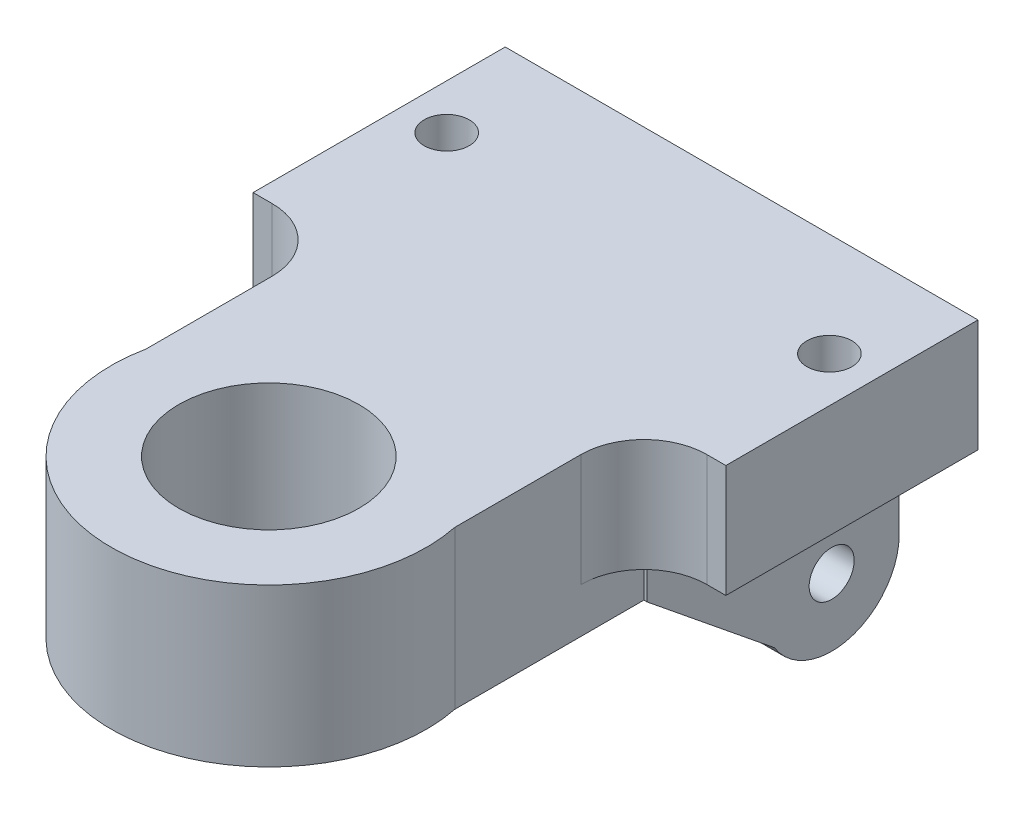
ISO-10303-21;
HEADER;
FILE_DESCRIPTION(('STEP AP214'),'2;1');
FILE_NAME('part.step','',(''),(''),'','','');
FILE_SCHEMA(('AUTOMOTIVE_DESIGN { 1 0 10303 214 1 1 1 1 }'));
ENDSEC;
DATA;
#1=APPLICATION_CONTEXT('core data for automotive mechanical design processes');
#2=APPLICATION_PROTOCOL_DEFINITION('international standard','automotive_design',2000,#1);
#3=PRODUCT_CONTEXT('',#1,'mechanical');
#4=PRODUCT('Part','Part','',(#3));
#5=PRODUCT_RELATED_PRODUCT_CATEGORY('part','',(#4));
#6=PRODUCT_DEFINITION_FORMATION('','',#4);
#7=PRODUCT_DEFINITION_CONTEXT('part definition',#1,'design');
#8=PRODUCT_DEFINITION('design','',#6,#7);
#9=PRODUCT_DEFINITION_SHAPE('','',#8);
#10=(LENGTH_UNIT() NAMED_UNIT(*) SI_UNIT(.MILLI.,.METRE.));
#11=(NAMED_UNIT(*) PLANE_ANGLE_UNIT() SI_UNIT($,.RADIAN.));
#12=(NAMED_UNIT(*) SI_UNIT($,.STERADIAN.) SOLID_ANGLE_UNIT());
#13=UNCERTAINTY_MEASURE_WITH_UNIT(LENGTH_MEASURE(1.E-05),#10,'distance_accuracy_value','');
#14=(GEOMETRIC_REPRESENTATION_CONTEXT(3) GLOBAL_UNCERTAINTY_ASSIGNED_CONTEXT((#13)) GLOBAL_UNIT_ASSIGNED_CONTEXT((#10,
#11,#12)) REPRESENTATION_CONTEXT('',''));
#15=CARTESIAN_POINT('',(0.,0.,0.));
#16=DIRECTION('',(0.,0.,1.));
#17=DIRECTION('',(1.,0.,0.));
#18=AXIS2_PLACEMENT_3D('',#15,#16,#17);
#19=CARTESIAN_POINT('',(0.,-22.5,0.));
#20=DIRECTION('',(0.,1.,0.));
#21=DIRECTION('',(0.,0.,1.));
#22=AXIS2_PLACEMENT_3D('',#19,#20,#21);
#23=PLANE('',#22);
#24=CARTESIAN_POINT('',(0.,-22.5,35.));
#25=DIRECTION('',(0.,1.,0.));
#26=DIRECTION('',(0.,0.,1.));
#27=AXIS2_PLACEMENT_3D('',#24,#25,#26);
#28=CIRCLE('',#27,20.);
#29=CARTESIAN_POINT('',(0.,-22.5,55.));
#30=VERTEX_POINT('',#29);
#31=EDGE_CURVE('E253',#30,#30,#28,.T.);
#32=ORIENTED_EDGE('',*,*,#31,.T.);
#33=EDGE_LOOP('',(#32));
#34=FACE_BOUND('',#33,.T.);
#35=DIRECTION('',(0.,0.,-1.));
#36=VECTOR('',#35,1.);
#37=CARTESIAN_POINT('',(-34.2928563989645,-22.5,-14.));
#38=LINE('',#37,#36);
#39=CARTESIAN_POINT('',(-34.2928563989645,-22.5,28.));
#40=VERTEX_POINT('',#39);
#41=CARTESIAN_POINT('',(-34.2928563989645,-22.5,-14.));
#42=VERTEX_POINT('',#41);
#43=EDGE_CURVE('E323',#40,#42,#38,.T.);
#44=ORIENTED_EDGE('',*,*,#43,.T.);
#45=DIRECTION('',(1.,0.,0.));
#46=VECTOR('',#45,1.);
#47=CARTESIAN_POINT('',(-35.,-22.5,-14.));
#48=LINE('',#47,#46);
#49=CARTESIAN_POINT('',(-20.,-22.5,-14.));
#50=VERTEX_POINT('',#49);
#51=EDGE_CURVE('E88',#42,#50,#48,.T.);
#52=ORIENTED_EDGE('',*,*,#51,.T.);
#53=DIRECTION('',(0.,0.,-1.));
#54=VECTOR('',#53,1.);
#55=CARTESIAN_POINT('',(-20.,-22.5,0.));
#56=LINE('',#55,#54);
#57=CARTESIAN_POINT('',(-20.,-22.5,-70.));
#58=VERTEX_POINT('',#57);
#59=EDGE_CURVE('E93',#50,#58,#56,.T.);
#60=ORIENTED_EDGE('',*,*,#59,.T.);
#61=DIRECTION('',(-1.,0.,0.));
#62=VECTOR('',#61,1.);
#63=CARTESIAN_POINT('',(0.,-22.5,-70.));
#64=LINE('',#63,#62);
#65=CARTESIAN_POINT('',(20.,-22.5,-70.));
#66=VERTEX_POINT('',#65);
#67=EDGE_CURVE('E361',#66,#58,#64,.T.);
#68=ORIENTED_EDGE('',*,*,#67,.F.);
#69=DIRECTION('',(0.,0.,-1.));
#70=VECTOR('',#69,1.);
#71=CARTESIAN_POINT('',(20.,-22.5,0.));
#72=LINE('',#71,#70);
#73=CARTESIAN_POINT('',(20.,-22.5,-14.));
#74=VERTEX_POINT('',#73);
#75=EDGE_CURVE('E271',#74,#66,#72,.T.);
#76=ORIENTED_EDGE('',*,*,#75,.F.);
#77=DIRECTION('',(-1.,0.,0.));
#78=VECTOR('',#77,1.);
#79=CARTESIAN_POINT('',(35.,-22.5,-14.));
#80=LINE('',#79,#78);
#81=CARTESIAN_POINT('',(34.2928563989645,-22.5,-14.));
#82=VERTEX_POINT('',#81);
#83=EDGE_CURVE('E12',#82,#74,#80,.T.);
#84=ORIENTED_EDGE('',*,*,#83,.F.);
#85=DIRECTION('',(0.,0.,1.));
#86=VECTOR('',#85,1.);
#87=CARTESIAN_POINT('',(34.2928563989645,-22.5,-14.));
#88=LINE('',#87,#86);
#89=CARTESIAN_POINT('',(34.2928563989645,-22.5,28.));
#90=VERTEX_POINT('',#89);
#91=EDGE_CURVE('E333',#82,#90,#88,.T.);
#92=ORIENTED_EDGE('',*,*,#91,.T.);
#93=CARTESIAN_POINT('',(0.,-22.5,35.));
#94=DIRECTION('',(0.,1.,0.));
#95=DIRECTION('',(0.,0.,1.));
#96=AXIS2_PLACEMENT_3D('',#93,#94,#95);
#97=CIRCLE('',#96,35.);
#98=EDGE_CURVE('E362',#40,#90,#97,.T.);
#99=ORIENTED_EDGE('',*,*,#98,.F.);
#100=EDGE_LOOP('',(#44,#52,#60,#68,#76,#84,#92,#99));
#101=FACE_BOUND('',#100,.T.);
#102=ADVANCED_FACE('F74',(#34,#101),#23,.F.);
#103=CARTESIAN_POINT('',(0.,-22.5,-14.));
#104=DIRECTION('',(0.,0.,-1.));
#105=DIRECTION('',(-1.,0.,0.));
#106=AXIS2_PLACEMENT_3D('',#103,#104,#105);
#107=PLANE('',#106);
#108=DIRECTION('',(-1.,0.,0.));
#109=VECTOR('',#108,1.);
#110=CARTESIAN_POINT('',(48.2928563989645,-12.5,-14.));
#111=LINE('',#110,#109);
#112=CARTESIAN_POINT('',(35.,-12.5,-14.));
#113=VERTEX_POINT('',#112);
#114=CARTESIAN_POINT('',(34.2928563989645,-12.5,-14.));
#115=VERTEX_POINT('',#114);
#116=EDGE_CURVE('E303',#113,#115,#111,.T.);
#117=ORIENTED_EDGE('',*,*,#116,.T.);
#118=DIRECTION('',(0.,1.,0.));
#119=VECTOR('',#118,1.);
#120=CARTESIAN_POINT('',(34.2928563989645,-22.5,-14.));
#121=LINE('',#120,#119);
#122=EDGE_CURVE('E350',#82,#115,#121,.T.);
#123=ORIENTED_EDGE('',*,*,#122,.F.);
#124=DIRECTION('',(-1.,0.,0.));
#125=VECTOR('',#124,1.);
#126=CARTESIAN_POINT('',(0.,-22.5,-14.));
#127=LINE('',#126,#125);
#128=CARTESIAN_POINT('',(35.,-22.5,-14.));
#129=VERTEX_POINT('',#128);
#130=EDGE_CURVE('E344',#129,#82,#127,.T.);
#131=ORIENTED_EDGE('',*,*,#130,.F.);
#132=DIRECTION('',(0.,1.,0.));
#133=VECTOR('',#132,1.);
#134=CARTESIAN_POINT('',(35.,-22.5,-14.));
#135=LINE('',#134,#133);
#136=EDGE_CURVE('E85',#129,#113,#135,.T.);
#137=ORIENTED_EDGE('',*,*,#136,.T.);
#138=EDGE_LOOP('',(#117,#123,#131,#137));
#139=FACE_BOUND('',#138,.T.);
#140=ADVANCED_FACE('F435',(#139),#107,.F.);
#141=CARTESIAN_POINT('',(0.,-22.5,-14.));
#142=DIRECTION('',(0.,0.,-1.));
#143=DIRECTION('',(-1.,0.,0.));
#144=AXIS2_PLACEMENT_3D('',#141,#142,#143);
#145=PLANE('',#144);
#146=DIRECTION('',(0.,1.,0.));
#147=VECTOR('',#146,1.);
#148=CARTESIAN_POINT('',(-48.2928563989645,-12.5,-14.));
#149=LINE('',#148,#147);
#150=CARTESIAN_POINT('',(-48.2928563989645,-12.5,-14.));
#151=VERTEX_POINT('',#150);
#152=CARTESIAN_POINT('',(-48.2928563989645,12.5,-14.));
#153=VERTEX_POINT('',#152);
#154=EDGE_CURVE('E324',#151,#153,#149,.T.);
#155=ORIENTED_EDGE('',*,*,#154,.T.);
#156=DIRECTION('',(-1.,0.,0.));
#157=VECTOR('',#156,1.);
#158=CARTESIAN_POINT('',(0.,12.5,-14.));
#159=LINE('',#158,#157);
#160=CARTESIAN_POINT('',(-52.5,12.5,-14.));
#161=VERTEX_POINT('',#160);
#162=EDGE_CURVE('E236',#153,#161,#159,.T.);
#163=ORIENTED_EDGE('',*,*,#162,.T.);
#164=DIRECTION('',(0.,1.,0.));
#165=VECTOR('',#164,1.);
#166=CARTESIAN_POINT('',(-52.5,-22.5,-14.));
#167=LINE('',#166,#165);
#168=CARTESIAN_POINT('',(-52.5,-12.5,-14.));
#169=VERTEX_POINT('',#168);
#170=EDGE_CURVE('E227',#169,#161,#167,.T.);
#171=ORIENTED_EDGE('',*,*,#170,.F.);
#172=DIRECTION('',(-1.,0.,0.));
#173=VECTOR('',#172,1.);
#174=CARTESIAN_POINT('',(0.,-12.5,-14.));
#175=LINE('',#174,#173);
#176=EDGE_CURVE('E228',#151,#169,#175,.T.);
#177=ORIENTED_EDGE('',*,*,#176,.F.);
#178=EDGE_LOOP('',(#155,#163,#171,#177));
#179=FACE_BOUND('',#178,.T.);
#180=ADVANCED_FACE('F437',(#179),#145,.F.);
#181=CARTESIAN_POINT('',(-34.2928563989645,12.5,-14.));
#182=DIRECTION('',(-1.,0.,0.));
#183=DIRECTION('',(0.,0.,1.));
#184=AXIS2_PLACEMENT_3D('',#181,#182,#183);
#185=PLANE('',#184);
#186=DIRECTION('',(0.,0.,-1.));
#187=VECTOR('',#186,1.);
#188=CARTESIAN_POINT('',(-34.2928563989645,12.5,-14.));
#189=LINE('',#188,#187);
#190=CARTESIAN_POINT('',(-34.2928563989645,12.5,28.));
#191=VERTEX_POINT('',#190);
#192=CARTESIAN_POINT('',(-34.2928563989645,12.5,0.));
#193=VERTEX_POINT('',#192);
#194=EDGE_CURVE('E330',#191,#193,#189,.T.);
#195=ORIENTED_EDGE('',*,*,#194,.T.);
#196=DIRECTION('',(0.,1.,0.));
#197=VECTOR('',#196,1.);
#198=CARTESIAN_POINT('',(-34.2928563989645,-12.5,0.));
#199=LINE('',#198,#197);
#200=CARTESIAN_POINT('',(-34.2928563989645,-12.5,0.));
#201=VERTEX_POINT('',#200);
#202=EDGE_CURVE('E318',#201,#193,#199,.T.);
#203=ORIENTED_EDGE('',*,*,#202,.F.);
#204=DIRECTION('',(0.,0.,-1.));
#205=VECTOR('',#204,1.);
#206=CARTESIAN_POINT('',(-34.2928563989645,-12.5,0.));
#207=LINE('',#206,#205);
#208=CARTESIAN_POINT('',(-34.2928563989645,-12.5,-14.));
#209=VERTEX_POINT('',#208);
#210=EDGE_CURVE('E320',#201,#209,#207,.T.);
#211=ORIENTED_EDGE('',*,*,#210,.T.);
#212=DIRECTION('',(0.,1.,0.));
#213=VECTOR('',#212,1.);
#214=CARTESIAN_POINT('',(-34.2928563989645,-22.5,-14.));
#215=LINE('',#214,#213);
#216=EDGE_CURVE('E232',#42,#209,#215,.T.);
#217=ORIENTED_EDGE('',*,*,#216,.F.);
#218=ORIENTED_EDGE('',*,*,#43,.F.);
#219=DIRECTION('',(0.,-1.,0.));
#220=VECTOR('',#219,1.);
#221=CARTESIAN_POINT('',(-34.2928563989645,12.5,28.));
#222=LINE('',#221,#220);
#223=EDGE_CURVE('E328',#191,#40,#222,.T.);
#224=ORIENTED_EDGE('',*,*,#223,.F.);
#225=EDGE_LOOP('',(#195,#203,#211,#217,#218,#224));
#226=FACE_BOUND('',#225,.T.);
#227=ADVANCED_FACE('F456',(#226),#185,.T.);
#228=CARTESIAN_POINT('',(0.,12.5,0.));
#229=DIRECTION('',(0.,1.,0.));
#230=DIRECTION('',(0.,0.,1.));
#231=AXIS2_PLACEMENT_3D('',#228,#229,#230);
#232=PLANE('',#231);
#233=CARTESIAN_POINT('',(-42.5,12.5,-47.));
#234=DIRECTION('',(0.,1.,0.));
#235=DIRECTION('',(0.,0.,1.));
#236=AXIS2_PLACEMENT_3D('',#233,#234,#235);
#237=CIRCLE('',#236,5.);
#238=CARTESIAN_POINT('',(-42.5,12.5,-42.));
#239=VERTEX_POINT('',#238);
#240=EDGE_CURVE('E402',#239,#239,#237,.T.);
#241=ORIENTED_EDGE('',*,*,#240,.F.);
#242=EDGE_LOOP('',(#241));
#243=FACE_BOUND('',#242,.T.);
#244=CARTESIAN_POINT('',(42.5,12.5,-47.));
#245=DIRECTION('',(0.,1.,0.));
#246=DIRECTION('',(0.,0.,1.));
#247=AXIS2_PLACEMENT_3D('',#244,#245,#246);
#248=CIRCLE('',#247,5.);
#249=CARTESIAN_POINT('',(42.5,12.5,-42.));
#250=VERTEX_POINT('',#249);
#251=EDGE_CURVE('E407',#250,#250,#248,.T.);
#252=ORIENTED_EDGE('',*,*,#251,.F.);
#253=EDGE_LOOP('',(#252));
#254=FACE_BOUND('',#253,.T.);
#255=CARTESIAN_POINT('',(0.,12.5,35.));
#256=DIRECTION('',(0.,1.,0.));
#257=DIRECTION('',(0.,0.,1.));
#258=AXIS2_PLACEMENT_3D('',#255,#256,#257);
#259=CIRCLE('',#258,20.);
#260=CARTESIAN_POINT('',(0.,12.5,55.));
#261=VERTEX_POINT('',#260);
#262=EDGE_CURVE('E412',#261,#261,#259,.T.);
#263=ORIENTED_EDGE('',*,*,#262,.F.);
#264=EDGE_LOOP('',(#263));
#265=FACE_BOUND('',#264,.T.);
#266=ORIENTED_EDGE('',*,*,#162,.F.);
#267=CARTESIAN_POINT('',(-48.2928563989645,12.5,0.));
#268=DIRECTION('',(0.,-1.,0.));
#269=DIRECTION('',(0.,0.,-1.));
#270=AXIS2_PLACEMENT_3D('',#267,#268,#269);
#271=CIRCLE('',#270,14.);
#272=EDGE_CURVE('E311',#153,#193,#271,.T.);
#273=ORIENTED_EDGE('',*,*,#272,.T.);
#274=ORIENTED_EDGE('',*,*,#194,.F.);
#275=CARTESIAN_POINT('',(0.,12.5,35.));
#276=DIRECTION('',(0.,1.,0.));
#277=DIRECTION('',(0.,0.,1.));
#278=AXIS2_PLACEMENT_3D('',#275,#276,#277);
#279=CIRCLE('',#278,35.);
#280=CARTESIAN_POINT('',(34.2928563989645,12.5,28.));
#281=VERTEX_POINT('',#280);
#282=EDGE_CURVE('E353',#191,#281,#279,.T.);
#283=ORIENTED_EDGE('',*,*,#282,.T.);
#284=DIRECTION('',(0.,0.,1.));
#285=VECTOR('',#284,1.);
#286=CARTESIAN_POINT('',(34.2928563989645,12.5,-14.));
#287=LINE('',#286,#285);
#288=CARTESIAN_POINT('',(34.2928563989645,12.5,0.));
#289=VERTEX_POINT('',#288);
#290=EDGE_CURVE('E335',#289,#281,#287,.T.);
#291=ORIENTED_EDGE('',*,*,#290,.F.);
#292=CARTESIAN_POINT('',(48.2928563989645,12.5,0.));
#293=DIRECTION('',(0.,-1.,0.));
#294=DIRECTION('',(0.,0.,1.));
#295=AXIS2_PLACEMENT_3D('',#292,#293,#294);
#296=CIRCLE('',#295,14.);
#297=CARTESIAN_POINT('',(48.2928563989645,12.5,-14.));
#298=VERTEX_POINT('',#297);
#299=EDGE_CURVE('E300',#289,#298,#296,.T.);
#300=ORIENTED_EDGE('',*,*,#299,.T.);
#301=DIRECTION('',(-1.,0.,0.));
#302=VECTOR('',#301,1.);
#303=CARTESIAN_POINT('',(0.,12.5,-14.));
#304=LINE('',#303,#302);
#305=CARTESIAN_POINT('',(52.5,12.5,-14.));
#306=VERTEX_POINT('',#305);
#307=EDGE_CURVE('E345',#306,#298,#304,.T.);
#308=ORIENTED_EDGE('',*,*,#307,.F.);
#309=DIRECTION('',(0.,0.,-1.));
#310=VECTOR('',#309,1.);
#311=CARTESIAN_POINT('',(52.5,12.5,-70.));
#312=LINE('',#311,#310);
#313=CARTESIAN_POINT('',(52.5,12.5,-70.));
#314=VERTEX_POINT('',#313);
#315=EDGE_CURVE('E372',#306,#314,#312,.T.);
#316=ORIENTED_EDGE('',*,*,#315,.T.);
#317=DIRECTION('',(-1.,0.,0.));
#318=VECTOR('',#317,1.);
#319=CARTESIAN_POINT('',(-52.5,12.5,-70.));
#320=LINE('',#319,#318);
#321=CARTESIAN_POINT('',(-52.5,12.5,-70.));
#322=VERTEX_POINT('',#321);
#323=EDGE_CURVE('E376',#314,#322,#320,.T.);
#324=ORIENTED_EDGE('',*,*,#323,.T.);
#325=DIRECTION('',(0.,0.,1.));
#326=VECTOR('',#325,1.);
#327=CARTESIAN_POINT('',(-52.5,12.5,-70.));
#328=LINE('',#327,#326);
#329=EDGE_CURVE('E378',#322,#161,#328,.T.);
#330=ORIENTED_EDGE('',*,*,#329,.T.);
#331=EDGE_LOOP('',(#266,#273,#274,#283,#291,#300,#308,#316,#324,#330));
#332=FACE_BOUND('',#331,.T.);
#333=ADVANCED_FACE('F457',(#243,#254,#265,#332),#232,.T.);
#334=CARTESIAN_POINT('',(0.,-12.5,0.));
#335=DIRECTION('',(0.,1.,0.));
#336=DIRECTION('',(0.,0.,1.));
#337=AXIS2_PLACEMENT_3D('',#334,#335,#336);
#338=PLANE('',#337);
#339=CARTESIAN_POINT('',(42.5,-12.5,-47.));
#340=DIRECTION('',(0.,1.,0.));
#341=DIRECTION('',(0.,0.,1.));
#342=AXIS2_PLACEMENT_3D('',#339,#340,#341);
#343=CIRCLE('',#342,5.);
#344=CARTESIAN_POINT('',(42.5,-12.5,-42.));
#345=VERTEX_POINT('',#344);
#346=EDGE_CURVE('E80',#345,#345,#343,.T.);
#347=ORIENTED_EDGE('',*,*,#346,.T.);
#348=EDGE_LOOP('',(#347));
#349=FACE_BOUND('',#348,.T.);
#350=DIRECTION('',(0.,0.,-1.));
#351=VECTOR('',#350,1.);
#352=CARTESIAN_POINT('',(52.5,-12.5,-70.));
#353=LINE('',#352,#351);
#354=CARTESIAN_POINT('',(52.5,-12.5,-14.));
#355=VERTEX_POINT('',#354);
#356=CARTESIAN_POINT('',(52.5,-12.5,-70.));
#357=VERTEX_POINT('',#356);
#358=EDGE_CURVE('E371',#355,#357,#353,.T.);
#359=ORIENTED_EDGE('',*,*,#358,.F.);
#360=DIRECTION('',(-1.,0.,0.));
#361=VECTOR('',#360,1.);
#362=CARTESIAN_POINT('',(0.,-12.5,-14.));
#363=LINE('',#362,#361);
#364=CARTESIAN_POINT('',(48.2928563989645,-12.5,-14.));
#365=VERTEX_POINT('',#364);
#366=EDGE_CURVE('E351',#355,#365,#363,.T.);
#367=ORIENTED_EDGE('',*,*,#366,.T.);
#368=CARTESIAN_POINT('',(48.2928563989645,-12.5,0.));
#369=DIRECTION('',(0.,-1.,0.));
#370=DIRECTION('',(0.,0.,1.));
#371=AXIS2_PLACEMENT_3D('',#368,#369,#370);
#372=CIRCLE('',#371,14.);
#373=CARTESIAN_POINT('',(34.2928563989645,-12.5,0.));
#374=VERTEX_POINT('',#373);
#375=EDGE_CURVE('E297',#374,#365,#372,.T.);
#376=ORIENTED_EDGE('',*,*,#375,.F.);
#377=DIRECTION('',(0.,0.,1.));
#378=VECTOR('',#377,1.);
#379=CARTESIAN_POINT('',(34.2928563989645,-12.5,-14.));
#380=LINE('',#379,#378);
#381=EDGE_CURVE('E296',#115,#374,#380,.T.);
#382=ORIENTED_EDGE('',*,*,#381,.F.);
#383=ORIENTED_EDGE('',*,*,#116,.F.);
#384=DIRECTION('',(0.,0.,-1.));
#385=VECTOR('',#384,1.);
#386=CARTESIAN_POINT('',(35.,-12.5,0.));
#387=LINE('',#386,#385);
#388=CARTESIAN_POINT('',(35.,-12.5,-70.));
#389=VERTEX_POINT('',#388);
#390=EDGE_CURVE('E397',#113,#389,#387,.T.);
#391=ORIENTED_EDGE('',*,*,#390,.T.);
#392=DIRECTION('',(-1.,0.,0.));
#393=VECTOR('',#392,1.);
#394=CARTESIAN_POINT('',(-52.5,-12.5,-70.));
#395=LINE('',#394,#393);
#396=EDGE_CURVE('E383',#357,#389,#395,.T.);
#397=ORIENTED_EDGE('',*,*,#396,.F.);
#398=EDGE_LOOP('',(#359,#367,#376,#382,#383,#391,#397));
#399=FACE_BOUND('',#398,.T.);
#400=ADVANCED_FACE('F460',(#349,#399),#338,.F.);
#401=CARTESIAN_POINT('',(52.5,12.5,-70.));
#402=DIRECTION('',(-1.,0.,0.));
#403=DIRECTION('',(0.,0.,1.));
#404=AXIS2_PLACEMENT_3D('',#401,#402,#403);
#405=PLANE('',#404);
#406=ORIENTED_EDGE('',*,*,#315,.F.);
#407=DIRECTION('',(0.,1.,0.));
#408=VECTOR('',#407,1.);
#409=CARTESIAN_POINT('',(52.5,-22.5,-14.));
#410=LINE('',#409,#408);
#411=EDGE_CURVE('E347',#355,#306,#410,.T.);
#412=ORIENTED_EDGE('',*,*,#411,.F.);
#413=ORIENTED_EDGE('',*,*,#358,.T.);
#414=DIRECTION('',(0.,-1.,0.));
#415=VECTOR('',#414,1.);
#416=CARTESIAN_POINT('',(52.5,12.5,-70.));
#417=LINE('',#416,#415);
#418=EDGE_CURVE('E394',#314,#357,#417,.T.);
#419=ORIENTED_EDGE('',*,*,#418,.F.);
#420=EDGE_LOOP('',(#406,#412,#413,#419));
#421=FACE_BOUND('',#420,.T.);
#422=ADVANCED_FACE('F75',(#421),#405,.F.);
#423=CARTESIAN_POINT('',(-52.5,12.5,-70.));
#424=DIRECTION('',(0.,0.,1.));
#425=DIRECTION('',(1.,0.,0.));
#426=AXIS2_PLACEMENT_3D('',#423,#424,#425);
#427=PLANE('',#426);
#428=ORIENTED_EDGE('',*,*,#396,.T.);
#429=DIRECTION('',(0.,1.,0.));
#430=VECTOR('',#429,1.);
#431=CARTESIAN_POINT('',(35.,-22.5,-70.));
#432=LINE('',#431,#430);
#433=CARTESIAN_POINT('',(35.,-37.5,-70.));
#434=VERTEX_POINT('',#433);
#435=EDGE_CURVE('E370',#434,#389,#432,.T.);
#436=ORIENTED_EDGE('',*,*,#435,.F.);
#437=DIRECTION('',(-1.,0.,0.));
#438=VECTOR('',#437,1.);
#439=CARTESIAN_POINT('',(35.,-37.5,-70.));
#440=LINE('',#439,#438);
#441=CARTESIAN_POINT('',(20.,-37.5,-70.));
#442=VERTEX_POINT('',#441);
#443=EDGE_CURVE('E276',#434,#442,#440,.T.);
#444=ORIENTED_EDGE('',*,*,#443,.T.);
#445=DIRECTION('',(0.,-1.,0.));
#446=VECTOR('',#445,1.);
#447=CARTESIAN_POINT('',(20.,0.,-70.));
#448=LINE('',#447,#446);
#449=EDGE_CURVE('E289',#66,#442,#448,.T.);
#450=ORIENTED_EDGE('',*,*,#449,.F.);
#451=ORIENTED_EDGE('',*,*,#67,.T.);
#452=DIRECTION('',(0.,-1.,0.));
#453=VECTOR('',#452,1.);
#454=CARTESIAN_POINT('',(-20.,0.,-70.));
#455=LINE('',#454,#453);
#456=CARTESIAN_POINT('',(-20.,-37.5,-70.));
#457=VERTEX_POINT('',#456);
#458=EDGE_CURVE('E256',#58,#457,#455,.T.);
#459=ORIENTED_EDGE('',*,*,#458,.T.);
#460=DIRECTION('',(1.,0.,0.));
#461=VECTOR('',#460,1.);
#462=CARTESIAN_POINT('',(-35.,-37.5,-70.));
#463=LINE('',#462,#461);
#464=CARTESIAN_POINT('',(-35.,-37.5,-70.));
#465=VERTEX_POINT('',#464);
#466=EDGE_CURVE('E263',#465,#457,#463,.T.);
#467=ORIENTED_EDGE('',*,*,#466,.F.);
#468=DIRECTION('',(0.,1.,0.));
#469=VECTOR('',#468,1.);
#470=CARTESIAN_POINT('',(-35.,-22.5,-70.));
#471=LINE('',#470,#469);
#472=CARTESIAN_POINT('',(-35.,-12.5,-70.));
#473=VERTEX_POINT('',#472);
#474=EDGE_CURVE('E368',#465,#473,#471,.T.);
#475=ORIENTED_EDGE('',*,*,#474,.T.);
#476=CARTESIAN_POINT('',(-52.5,-12.5,-70.));
#477=VERTEX_POINT('',#476);
#478=EDGE_CURVE('E381',#473,#477,#395,.T.);
#479=ORIENTED_EDGE('',*,*,#478,.T.);
#480=DIRECTION('',(0.,-1.,0.));
#481=VECTOR('',#480,1.);
#482=CARTESIAN_POINT('',(-52.5,12.5,-70.));
#483=LINE('',#482,#481);
#484=EDGE_CURVE('E385',#322,#477,#483,.T.);
#485=ORIENTED_EDGE('',*,*,#484,.F.);
#486=ORIENTED_EDGE('',*,*,#323,.F.);
#487=ORIENTED_EDGE('',*,*,#418,.T.);
#488=EDGE_LOOP('',(#428,#436,#444,#450,#451,#459,#467,#475,#479,#485,#486,#487));
#489=FACE_BOUND('',#488,.T.);
#490=ADVANCED_FACE('F465',(#489),#427,.F.);
#491=CARTESIAN_POINT('',(-52.5,12.5,-70.));
#492=DIRECTION('',(1.,0.,0.));
#493=DIRECTION('',(0.,0.,-1.));
#494=AXIS2_PLACEMENT_3D('',#491,#492,#493);
#495=PLANE('',#494);
#496=DIRECTION('',(0.,0.,1.));
#497=VECTOR('',#496,1.);
#498=CARTESIAN_POINT('',(-52.5,-12.5,-70.));
#499=LINE('',#498,#497);
#500=EDGE_CURVE('E380',#477,#169,#499,.T.);
#501=ORIENTED_EDGE('',*,*,#500,.T.);
#502=ORIENTED_EDGE('',*,*,#170,.T.);
#503=ORIENTED_EDGE('',*,*,#329,.F.);
#504=ORIENTED_EDGE('',*,*,#484,.T.);
#505=EDGE_LOOP('',(#501,#502,#503,#504));
#506=FACE_BOUND('',#505,.T.);
#507=ADVANCED_FACE('F464',(#506),#495,.F.);
#508=CARTESIAN_POINT('',(-42.5,-12.5,-47.));
#509=DIRECTION('',(0.,1.,0.));
#510=DIRECTION('',(0.,0.,1.));
#511=AXIS2_PLACEMENT_3D('',#508,#509,#510);
#512=CIRCLE('',#511,5.);
#513=CARTESIAN_POINT('',(-42.5,-12.5,-42.));
#514=VERTEX_POINT('',#513);
#515=EDGE_CURVE('E398',#514,#514,#512,.T.);
#516=ORIENTED_EDGE('',*,*,#515,.T.);
#517=EDGE_LOOP('',(#516));
#518=FACE_BOUND('',#517,.T.);
#519=DIRECTION('',(0.,0.,-1.));
#520=VECTOR('',#519,1.);
#521=CARTESIAN_POINT('',(-35.,-12.5,0.));
#522=LINE('',#521,#520);
#523=CARTESIAN_POINT('',(-35.,-12.5,-14.));
#524=VERTEX_POINT('',#523);
#525=EDGE_CURVE('E393',#524,#473,#522,.T.);
#526=ORIENTED_EDGE('',*,*,#525,.F.);
#527=DIRECTION('',(-1.,0.,0.));
#528=VECTOR('',#527,1.);
#529=CARTESIAN_POINT('',(-34.2928563989645,-12.5,-14.));
#530=LINE('',#529,#528);
#531=EDGE_CURVE('E222',#209,#524,#530,.T.);
#532=ORIENTED_EDGE('',*,*,#531,.F.);
#533=ORIENTED_EDGE('',*,*,#210,.F.);
#534=CARTESIAN_POINT('',(-48.2928563989645,-12.5,0.));
#535=DIRECTION('',(0.,-1.,0.));
#536=DIRECTION('',(0.,0.,-1.));
#537=AXIS2_PLACEMENT_3D('',#534,#535,#536);
#538=CIRCLE('',#537,14.);
#539=EDGE_CURVE('E313',#151,#201,#538,.T.);
#540=ORIENTED_EDGE('',*,*,#539,.F.);
#541=ORIENTED_EDGE('',*,*,#176,.T.);
#542=ORIENTED_EDGE('',*,*,#500,.F.);
#543=ORIENTED_EDGE('',*,*,#478,.F.);
#544=EDGE_LOOP('',(#526,#532,#533,#540,#541,#542,#543));
#545=FACE_BOUND('',#544,.T.);
#546=ADVANCED_FACE('F451',(#518,#545),#338,.F.);
#547=CARTESIAN_POINT('',(35.,-22.5,0.));
#548=DIRECTION('',(1.,0.,0.));
#549=DIRECTION('',(0.,0.,-1.));
#550=AXIS2_PLACEMENT_3D('',#547,#548,#549);
#551=PLANE('',#550);
#552=ORIENTED_EDGE('',*,*,#136,.F.);
#553=DIRECTION('',(0.,-0.629796155832871,-0.776760453484945));
#554=VECTOR('',#553,1.);
#555=CARTESIAN_POINT('',(35.,-6.72671758069868,5.45401205054981));
#556=LINE('',#555,#554);
#557=CARTESIAN_POINT('',(35.,-45.4084080451959,-42.2541347021601));
#558=VERTEX_POINT('',#557);
#559=EDGE_CURVE('E275',#129,#558,#556,.T.);
#560=ORIENTED_EDGE('',*,*,#559,.T.);
#561=CARTESIAN_POINT('',(35.,-37.5,-55.));
#562=DIRECTION('',(1.,0.,0.));
#563=DIRECTION('',(0.,0.,-1.));
#564=AXIS2_PLACEMENT_3D('',#561,#562,#563);
#565=CIRCLE('',#564,15.);
#566=EDGE_CURVE('E277',#558,#434,#565,.T.);
#567=ORIENTED_EDGE('',*,*,#566,.T.);
#568=ORIENTED_EDGE('',*,*,#435,.T.);
#569=ORIENTED_EDGE('',*,*,#390,.F.);
#570=EDGE_LOOP('',(#552,#560,#567,#568,#569));
#571=FACE_BOUND('',#570,.T.);
#572=CARTESIAN_POINT('',(35.,-37.5,-55.));
#573=DIRECTION('',(1.,0.,0.));
#574=DIRECTION('',(0.,0.,-1.));
#575=AXIS2_PLACEMENT_3D('',#572,#573,#574);
#576=CIRCLE('',#575,5.);
#577=CARTESIAN_POINT('',(35.,-37.5,-60.));
#578=VERTEX_POINT('',#577);
#579=EDGE_CURVE('E268',#578,#578,#576,.T.);
#580=ORIENTED_EDGE('',*,*,#579,.F.);
#581=EDGE_LOOP('',(#580));
#582=FACE_BOUND('',#581,.T.);
#583=ADVANCED_FACE('F449',(#571,#582),#551,.T.);
#584=CARTESIAN_POINT('',(0.,-22.5,35.));
#585=DIRECTION('',(0.,1.,0.));
#586=DIRECTION('',(0.,0.,1.));
#587=AXIS2_PLACEMENT_3D('',#584,#585,#586);
#588=CYLINDRICAL_SURFACE('',#587,35.);
#589=ORIENTED_EDGE('',*,*,#223,.T.);
#590=ORIENTED_EDGE('',*,*,#98,.T.);
#591=DIRECTION('',(0.,-1.,0.));
#592=VECTOR('',#591,1.);
#593=CARTESIAN_POINT('',(34.2928563989645,12.5,28.));
#594=LINE('',#593,#592);
#595=EDGE_CURVE('E340',#281,#90,#594,.T.);
#596=ORIENTED_EDGE('',*,*,#595,.F.);
#597=ORIENTED_EDGE('',*,*,#282,.F.);
#598=EDGE_LOOP('',(#589,#590,#596,#597));
#599=FACE_BOUND('',#598,.T.);
#600=ADVANCED_FACE('F444',(#599),#588,.T.);
#601=CARTESIAN_POINT('',(-35.,-22.5,0.));
#602=DIRECTION('',(1.,0.,0.));
#603=DIRECTION('',(0.,0.,-1.));
#604=AXIS2_PLACEMENT_3D('',#601,#602,#603);
#605=PLANE('',#604);
#606=ORIENTED_EDGE('',*,*,#474,.F.);
#607=CARTESIAN_POINT('',(-35.,-37.5,-55.));
#608=DIRECTION('',(1.,0.,0.));
#609=DIRECTION('',(0.,0.,-1.));
#610=AXIS2_PLACEMENT_3D('',#607,#608,#609);
#611=CIRCLE('',#610,15.);
#612=CARTESIAN_POINT('',(-35.,-45.4084080451959,-42.2541347021601));
#613=VERTEX_POINT('',#612);
#614=EDGE_CURVE('E241',#613,#465,#611,.T.);
#615=ORIENTED_EDGE('',*,*,#614,.F.);
#616=DIRECTION('',(0.,-0.629796155832871,-0.776760453484945));
#617=VECTOR('',#616,1.);
#618=CARTESIAN_POINT('',(-35.,-6.72671758069868,5.45401205054981));
#619=LINE('',#618,#617);
#620=CARTESIAN_POINT('',(-35.,-22.5,-14.));
#621=VERTEX_POINT('',#620);
#622=EDGE_CURVE('E231',#621,#613,#619,.T.);
#623=ORIENTED_EDGE('',*,*,#622,.F.);
#624=DIRECTION('',(0.,1.,0.));
#625=VECTOR('',#624,1.);
#626=CARTESIAN_POINT('',(-35.,-22.5,-14.));
#627=LINE('',#626,#625);
#628=EDGE_CURVE('E217',#621,#524,#627,.T.);
#629=ORIENTED_EDGE('',*,*,#628,.T.);
#630=ORIENTED_EDGE('',*,*,#525,.T.);
#631=EDGE_LOOP('',(#606,#615,#623,#629,#630));
#632=FACE_BOUND('',#631,.T.);
#633=CARTESIAN_POINT('',(-35.,-37.5,-55.));
#634=DIRECTION('',(1.,0.,0.));
#635=DIRECTION('',(0.,0.,-1.));
#636=AXIS2_PLACEMENT_3D('',#633,#634,#635);
#637=CIRCLE('',#636,5.);
#638=CARTESIAN_POINT('',(-35.,-37.5,-60.));
#639=VERTEX_POINT('',#638);
#640=EDGE_CURVE('E245',#639,#639,#637,.T.);
#641=ORIENTED_EDGE('',*,*,#640,.T.);
#642=EDGE_LOOP('',(#641));
#643=FACE_BOUND('',#642,.T.);
#644=ADVANCED_FACE('F238',(#632,#643),#605,.F.);
#645=ORIENTED_EDGE('',*,*,#216,.T.);
#646=ORIENTED_EDGE('',*,*,#531,.T.);
#647=ORIENTED_EDGE('',*,*,#628,.F.);
#648=DIRECTION('',(-1.,0.,0.));
#649=VECTOR('',#648,1.);
#650=CARTESIAN_POINT('',(0.,-22.5,-14.));
#651=LINE('',#650,#649);
#652=EDGE_CURVE('E218',#42,#621,#651,.T.);
#653=ORIENTED_EDGE('',*,*,#652,.F.);
#654=EDGE_LOOP('',(#645,#646,#647,#653));
#655=FACE_BOUND('',#654,.T.);
#656=ADVANCED_FACE('F216',(#655),#145,.F.);
#657=ORIENTED_EDGE('',*,*,#307,.T.);
#658=DIRECTION('',(0.,1.,0.));
#659=VECTOR('',#658,1.);
#660=CARTESIAN_POINT('',(48.2928563989645,-12.5,-14.));
#661=LINE('',#660,#659);
#662=EDGE_CURVE('E308',#365,#298,#661,.T.);
#663=ORIENTED_EDGE('',*,*,#662,.F.);
#664=ORIENTED_EDGE('',*,*,#366,.F.);
#665=ORIENTED_EDGE('',*,*,#411,.T.);
#666=EDGE_LOOP('',(#657,#663,#664,#665));
#667=FACE_BOUND('',#666,.T.);
#668=ADVANCED_FACE('F445',(#667),#107,.F.);
#669=CARTESIAN_POINT('',(34.2928563989645,12.5,-14.));
#670=DIRECTION('',(1.,0.,0.));
#671=DIRECTION('',(0.,0.,-1.));
#672=AXIS2_PLACEMENT_3D('',#669,#670,#671);
#673=PLANE('',#672);
#674=DIRECTION('',(0.,1.,0.));
#675=VECTOR('',#674,1.);
#676=CARTESIAN_POINT('',(34.2928563989645,-12.5,0.));
#677=LINE('',#676,#675);
#678=EDGE_CURVE('E304',#374,#289,#677,.T.);
#679=ORIENTED_EDGE('',*,*,#678,.T.);
#680=ORIENTED_EDGE('',*,*,#290,.T.);
#681=ORIENTED_EDGE('',*,*,#595,.T.);
#682=ORIENTED_EDGE('',*,*,#91,.F.);
#683=ORIENTED_EDGE('',*,*,#122,.T.);
#684=ORIENTED_EDGE('',*,*,#381,.T.);
#685=EDGE_LOOP('',(#679,#680,#681,#682,#683,#684));
#686=FACE_BOUND('',#685,.T.);
#687=ADVANCED_FACE('F497',(#686),#673,.T.);
#688=CARTESIAN_POINT('',(-48.2928563989645,-12.5,0.));
#689=DIRECTION('',(0.,1.,0.));
#690=DIRECTION('',(0.,0.,1.));
#691=AXIS2_PLACEMENT_3D('',#688,#689,#690);
#692=CYLINDRICAL_SURFACE('',#691,14.);
#693=ORIENTED_EDGE('',*,*,#272,.F.);
#694=ORIENTED_EDGE('',*,*,#154,.F.);
#695=ORIENTED_EDGE('',*,*,#539,.T.);
#696=ORIENTED_EDGE('',*,*,#202,.T.);
#697=EDGE_LOOP('',(#693,#694,#695,#696));
#698=FACE_BOUND('',#697,.T.);
#699=ADVANCED_FACE('F512',(#698),#692,.F.);
#700=CARTESIAN_POINT('',(48.2928563989645,-12.5,0.));
#701=DIRECTION('',(0.,1.,0.));
#702=DIRECTION('',(0.,0.,1.));
#703=AXIS2_PLACEMENT_3D('',#700,#701,#702);
#704=CYLINDRICAL_SURFACE('',#703,14.);
#705=ORIENTED_EDGE('',*,*,#299,.F.);
#706=ORIENTED_EDGE('',*,*,#678,.F.);
#707=ORIENTED_EDGE('',*,*,#375,.T.);
#708=ORIENTED_EDGE('',*,*,#662,.T.);
#709=EDGE_LOOP('',(#705,#706,#707,#708));
#710=FACE_BOUND('',#709,.T.);
#711=ADVANCED_FACE('F547',(#710),#704,.F.);
#712=CARTESIAN_POINT('',(35.,-6.72671758069868,5.45401205054981));
#713=DIRECTION('',(0.,0.776760453484945,-0.629796155832871));
#714=DIRECTION('',(0.,0.629796155832871,0.776760453484945));
#715=AXIS2_PLACEMENT_3D('',#712,#713,#714);
#716=PLANE('',#715);
#717=DIRECTION('',(0.,-0.629796155832871,-0.776760453484945));
#718=VECTOR('',#717,1.);
#719=CARTESIAN_POINT('',(20.,-6.72671758069868,5.45401205054981));
#720=LINE('',#719,#718);
#721=CARTESIAN_POINT('',(20.,-45.4084080451959,-42.2541347021601));
#722=VERTEX_POINT('',#721);
#723=EDGE_CURVE('E284',#74,#722,#720,.T.);
#724=ORIENTED_EDGE('',*,*,#723,.T.);
#725=DIRECTION('',(-1.,0.,0.));
#726=VECTOR('',#725,1.);
#727=CARTESIAN_POINT('',(35.,-45.4084080451959,-42.2541347021601));
#728=LINE('',#727,#726);
#729=EDGE_CURVE('E295',#558,#722,#728,.T.);
#730=ORIENTED_EDGE('',*,*,#729,.F.);
#731=ORIENTED_EDGE('',*,*,#559,.F.);
#732=ORIENTED_EDGE('',*,*,#130,.T.);
#733=ORIENTED_EDGE('',*,*,#83,.T.);
#734=EDGE_LOOP('',(#724,#730,#731,#732,#733));
#735=FACE_BOUND('',#734,.T.);
#736=ADVANCED_FACE('F496',(#735),#716,.F.);
#737=CARTESIAN_POINT('',(35.,-37.5,-55.));
#738=DIRECTION('',(-1.,0.,0.));
#739=DIRECTION('',(0.,0.,1.));
#740=AXIS2_PLACEMENT_3D('',#737,#738,#739);
#741=CYLINDRICAL_SURFACE('',#740,15.);
#742=CARTESIAN_POINT('',(20.,-37.5,-55.));
#743=DIRECTION('',(1.,0.,0.));
#744=DIRECTION('',(0.,0.,-1.));
#745=AXIS2_PLACEMENT_3D('',#742,#743,#744);
#746=CIRCLE('',#745,15.);
#747=EDGE_CURVE('E283',#722,#442,#746,.T.);
#748=ORIENTED_EDGE('',*,*,#747,.T.);
#749=ORIENTED_EDGE('',*,*,#443,.F.);
#750=ORIENTED_EDGE('',*,*,#566,.F.);
#751=ORIENTED_EDGE('',*,*,#729,.T.);
#752=EDGE_LOOP('',(#748,#749,#750,#751));
#753=FACE_BOUND('',#752,.T.);
#754=ADVANCED_FACE('F486',(#753),#741,.T.);
#755=CARTESIAN_POINT('',(35.,-37.5,-55.));
#756=DIRECTION('',(-1.,0.,0.));
#757=DIRECTION('',(0.,0.,1.));
#758=AXIS2_PLACEMENT_3D('',#755,#756,#757);
#759=CYLINDRICAL_SURFACE('',#758,5.);
#760=ORIENTED_EDGE('',*,*,#579,.T.);
#761=EDGE_LOOP('',(#760));
#762=FACE_BOUND('',#761,.T.);
#763=CARTESIAN_POINT('',(20.,-37.5,-55.));
#764=DIRECTION('',(1.,0.,0.));
#765=DIRECTION('',(0.,0.,-1.));
#766=AXIS2_PLACEMENT_3D('',#763,#764,#765);
#767=CIRCLE('',#766,5.);
#768=CARTESIAN_POINT('',(20.,-37.5,-60.));
#769=VERTEX_POINT('',#768);
#770=EDGE_CURVE('E269',#769,#769,#767,.T.);
#771=ORIENTED_EDGE('',*,*,#770,.F.);
#772=EDGE_LOOP('',(#771));
#773=FACE_BOUND('',#772,.T.);
#774=ADVANCED_FACE('F542',(#762,#773),#759,.F.);
#775=CARTESIAN_POINT('',(20.,0.,0.));
#776=DIRECTION('',(1.,0.,0.));
#777=DIRECTION('',(0.,0.,-1.));
#778=AXIS2_PLACEMENT_3D('',#775,#776,#777);
#779=PLANE('',#778);
#780=ORIENTED_EDGE('',*,*,#770,.T.);
#781=EDGE_LOOP('',(#780));
#782=FACE_BOUND('',#781,.T.);
#783=ORIENTED_EDGE('',*,*,#723,.F.);
#784=ORIENTED_EDGE('',*,*,#75,.T.);
#785=ORIENTED_EDGE('',*,*,#449,.T.);
#786=ORIENTED_EDGE('',*,*,#747,.F.);
#787=EDGE_LOOP('',(#783,#784,#785,#786));
#788=FACE_BOUND('',#787,.T.);
#789=ADVANCED_FACE('F491',(#782,#788),#779,.F.);
#790=CARTESIAN_POINT('',(-35.,-6.72671758069868,5.45401205054981));
#791=DIRECTION('',(0.,-0.776760453484945,0.629796155832871));
#792=DIRECTION('',(0.,-0.629796155832871,-0.776760453484945));
#793=AXIS2_PLACEMENT_3D('',#790,#791,#792);
#794=PLANE('',#793);
#795=DIRECTION('',(0.,-0.629796155832871,-0.776760453484945));
#796=VECTOR('',#795,1.);
#797=CARTESIAN_POINT('',(-20.,-6.72671758069868,5.45401205054981));
#798=LINE('',#797,#796);
#799=CARTESIAN_POINT('',(-20.,-45.4084080451959,-42.2541347021601));
#800=VERTEX_POINT('',#799);
#801=EDGE_CURVE('E251',#50,#800,#798,.T.);
#802=ORIENTED_EDGE('',*,*,#801,.F.);
#803=ORIENTED_EDGE('',*,*,#51,.F.);
#804=ORIENTED_EDGE('',*,*,#652,.T.);
#805=ORIENTED_EDGE('',*,*,#622,.T.);
#806=DIRECTION('',(1.,0.,0.));
#807=VECTOR('',#806,1.);
#808=CARTESIAN_POINT('',(-35.,-45.4084080451959,-42.2541347021601));
#809=LINE('',#808,#807);
#810=EDGE_CURVE('E242',#613,#800,#809,.T.);
#811=ORIENTED_EDGE('',*,*,#810,.T.);
#812=EDGE_LOOP('',(#802,#803,#804,#805,#811));
#813=FACE_BOUND('',#812,.T.);
#814=ADVANCED_FACE('F235',(#813),#794,.T.);
#815=CARTESIAN_POINT('',(-35.,-37.5,-55.));
#816=DIRECTION('',(1.,0.,0.));
#817=DIRECTION('',(0.,0.,-1.));
#818=AXIS2_PLACEMENT_3D('',#815,#816,#817);
#819=CYLINDRICAL_SURFACE('',#818,5.);
#820=ORIENTED_EDGE('',*,*,#640,.F.);
#821=EDGE_LOOP('',(#820));
#822=FACE_BOUND('',#821,.T.);
#823=CARTESIAN_POINT('',(-20.,-37.5,-55.));
#824=DIRECTION('',(1.,0.,0.));
#825=DIRECTION('',(0.,0.,-1.));
#826=AXIS2_PLACEMENT_3D('',#823,#824,#825);
#827=CIRCLE('',#826,5.);
#828=CARTESIAN_POINT('',(-20.,-37.5,-60.));
#829=VERTEX_POINT('',#828);
#830=EDGE_CURVE('E252',#829,#829,#827,.T.);
#831=ORIENTED_EDGE('',*,*,#830,.T.);
#832=EDGE_LOOP('',(#831));
#833=FACE_BOUND('',#832,.T.);
#834=ADVANCED_FACE('F530',(#822,#833),#819,.F.);
#835=CARTESIAN_POINT('',(-35.,-37.5,-55.));
#836=DIRECTION('',(1.,0.,0.));
#837=DIRECTION('',(0.,0.,-1.));
#838=AXIS2_PLACEMENT_3D('',#835,#836,#837);
#839=CYLINDRICAL_SURFACE('',#838,15.);
#840=CARTESIAN_POINT('',(-20.,-37.5,-55.));
#841=DIRECTION('',(1.,0.,0.));
#842=DIRECTION('',(0.,0.,-1.));
#843=AXIS2_PLACEMENT_3D('',#840,#841,#842);
#844=CIRCLE('',#843,15.);
#845=EDGE_CURVE('E250',#800,#457,#844,.T.);
#846=ORIENTED_EDGE('',*,*,#845,.F.);
#847=ORIENTED_EDGE('',*,*,#810,.F.);
#848=ORIENTED_EDGE('',*,*,#614,.T.);
#849=ORIENTED_EDGE('',*,*,#466,.T.);
#850=EDGE_LOOP('',(#846,#847,#848,#849));
#851=FACE_BOUND('',#850,.T.);
#852=ADVANCED_FACE('F522',(#851),#839,.T.);
#853=CARTESIAN_POINT('',(-20.,0.,0.));
#854=DIRECTION('',(-1.,0.,0.));
#855=DIRECTION('',(0.,0.,-1.));
#856=AXIS2_PLACEMENT_3D('',#853,#854,#855);
#857=PLANE('',#856);
#858=ORIENTED_EDGE('',*,*,#830,.F.);
#859=EDGE_LOOP('',(#858));
#860=FACE_BOUND('',#859,.T.);
#861=ORIENTED_EDGE('',*,*,#801,.T.);
#862=ORIENTED_EDGE('',*,*,#845,.T.);
#863=ORIENTED_EDGE('',*,*,#458,.F.);
#864=ORIENTED_EDGE('',*,*,#59,.F.);
#865=EDGE_LOOP('',(#861,#862,#863,#864));
#866=FACE_BOUND('',#865,.T.);
#867=ADVANCED_FACE('F525',(#860,#866),#857,.F.);
#868=CARTESIAN_POINT('',(-42.5,-52.5,-47.));
#869=DIRECTION('',(0.,1.,0.));
#870=DIRECTION('',(0.,0.,1.));
#871=AXIS2_PLACEMENT_3D('',#868,#869,#870);
#872=CYLINDRICAL_SURFACE('',#871,5.);
#873=ORIENTED_EDGE('',*,*,#240,.T.);
#874=EDGE_LOOP('',(#873));
#875=FACE_BOUND('',#874,.T.);
#876=ORIENTED_EDGE('',*,*,#515,.F.);
#877=EDGE_LOOP('',(#876));
#878=FACE_BOUND('',#877,.T.);
#879=ADVANCED_FACE('F430',(#875,#878),#872,.F.);
#880=CARTESIAN_POINT('',(42.5,-52.5,-47.));
#881=DIRECTION('',(0.,1.,0.));
#882=DIRECTION('',(0.,0.,1.));
#883=AXIS2_PLACEMENT_3D('',#880,#881,#882);
#884=CYLINDRICAL_SURFACE('',#883,5.);
#885=ORIENTED_EDGE('',*,*,#251,.T.);
#886=EDGE_LOOP('',(#885));
#887=FACE_BOUND('',#886,.T.);
#888=ORIENTED_EDGE('',*,*,#346,.F.);
#889=EDGE_LOOP('',(#888));
#890=FACE_BOUND('',#889,.T.);
#891=ADVANCED_FACE('F423',(#887,#890),#884,.F.);
#892=CARTESIAN_POINT('',(0.,-52.5,35.));
#893=DIRECTION('',(0.,1.,0.));
#894=DIRECTION('',(0.,0.,1.));
#895=AXIS2_PLACEMENT_3D('',#892,#893,#894);
#896=CYLINDRICAL_SURFACE('',#895,20.);
#897=ORIENTED_EDGE('',*,*,#262,.T.);
#898=EDGE_LOOP('',(#897));
#899=FACE_BOUND('',#898,.T.);
#900=ORIENTED_EDGE('',*,*,#31,.F.);
#901=EDGE_LOOP('',(#900));
#902=FACE_BOUND('',#901,.T.);
#903=ADVANCED_FACE('F418',(#899,#902),#896,.F.);
#904=CLOSED_SHELL('',(#102,#140,#180,#227,#333,#400,#422,#490,#507,#546,#583,#600,#644,#656,
#668,#687,#699,#711,#736,#754,#774,#789,#814,#834,#852,#867,#879,#891,#903));
#905=MANIFOLD_SOLID_BREP('B2',#904);
#906=ADVANCED_BREP_SHAPE_REPRESENTATION('',(#18,#905),#14);
#907=SHAPE_DEFINITION_REPRESENTATION(#9,#906);
ENDSEC;
END-ISO-10303-21;
